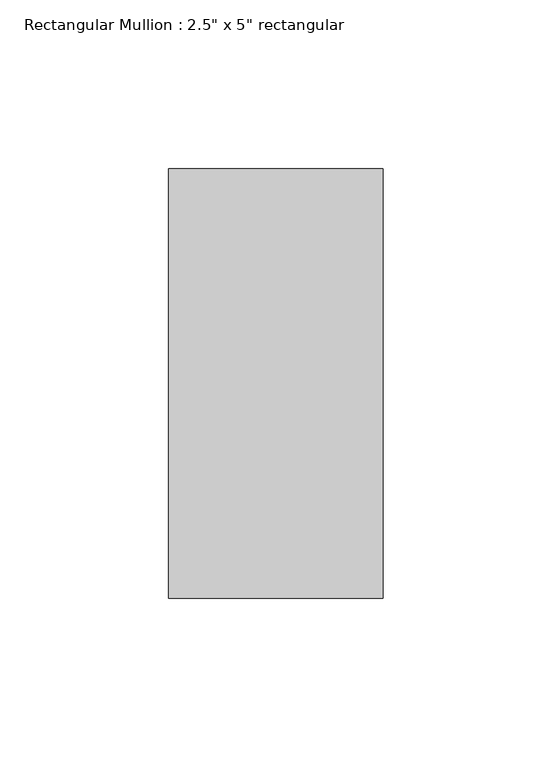
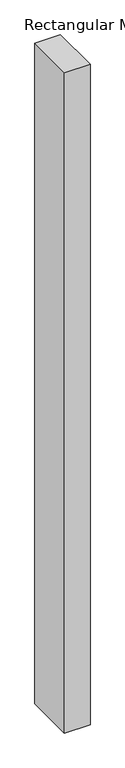
"""IFC4 building model written with IfcOpenShell, lengths in millimetres: member geometry."""

from ifc_helpers import new_model, si_unit, frame, origin, place, context, project, spatial, polyline, outline, extrude, source, transform, mapped, element, save


def member_64ee9188(model_context):
    return source(origin(), model_context, "Body", "SweptSolid", [
        extrude(outline(polyline([(0.0, 63.5), (0.0, -63.5), (-63.5, -63.5), (-63.5, 63.5), (0.0, 63.5)])), frame((0.0, 0.0, -1733.55), z_axis=(0.0, 0.0, 1.0), x_axis=(1.0, 0.0, 0.0)), (0.0, 0.0, 1.0), 1733.55),
    ])


if __name__ == "__main__":
    model = new_model("IFC4")
    model_context = context("Model", 3, world=origin())
    ifc_project = project(units=[si_unit("LENGTHUNIT", "METRE", prefix="MILLI")], contexts=[model_context])
    site = spatial("IfcSite", under=ifc_project)
    building = spatial("IfcBuilding", under=site)
    placement = place(None, origin())
    member_shape = member_64ee9188(model_context)
    element("IfcMember", 1, ObjectType="Rectangular Mullion : 2.5\" x 5\" rectangular", at=placement, inside=building, context=model_context, shape_type="MappedRepresentation", body=[
        mapped(member_shape, transform((0.0, 0.0, 0.0), x_axis=(1.0, 0.0, 0.0), y_axis=(0.0, 1.0, 0.0), z_axis=(0.0, 0.0, 1.0))),
    ])
    save(model, "model.ifc")

# Revit data of these elements
# Type "Rectangular Mullion : 2.5\" x 5\" rectangular"
#   built-in parameter 1007304 = 0.416667 (stored number, unit not read)
#   built-in parameter 1007301 = 0.104167 (stored number, unit not read)
#   built-in parameter 1007300 = 0.104167 (stored number, unit not read)
# Element 1 (IfcMember, "Rectangular Mullion : 2.5\" x 5\" rectangular")
#   Materials on its faces: "Aluminum"
# Materials
#   "Aluminum": class "Metal", colour RGB 247 247 247, transparency 0, Description = "Aluminum 6061", Cost = 0
